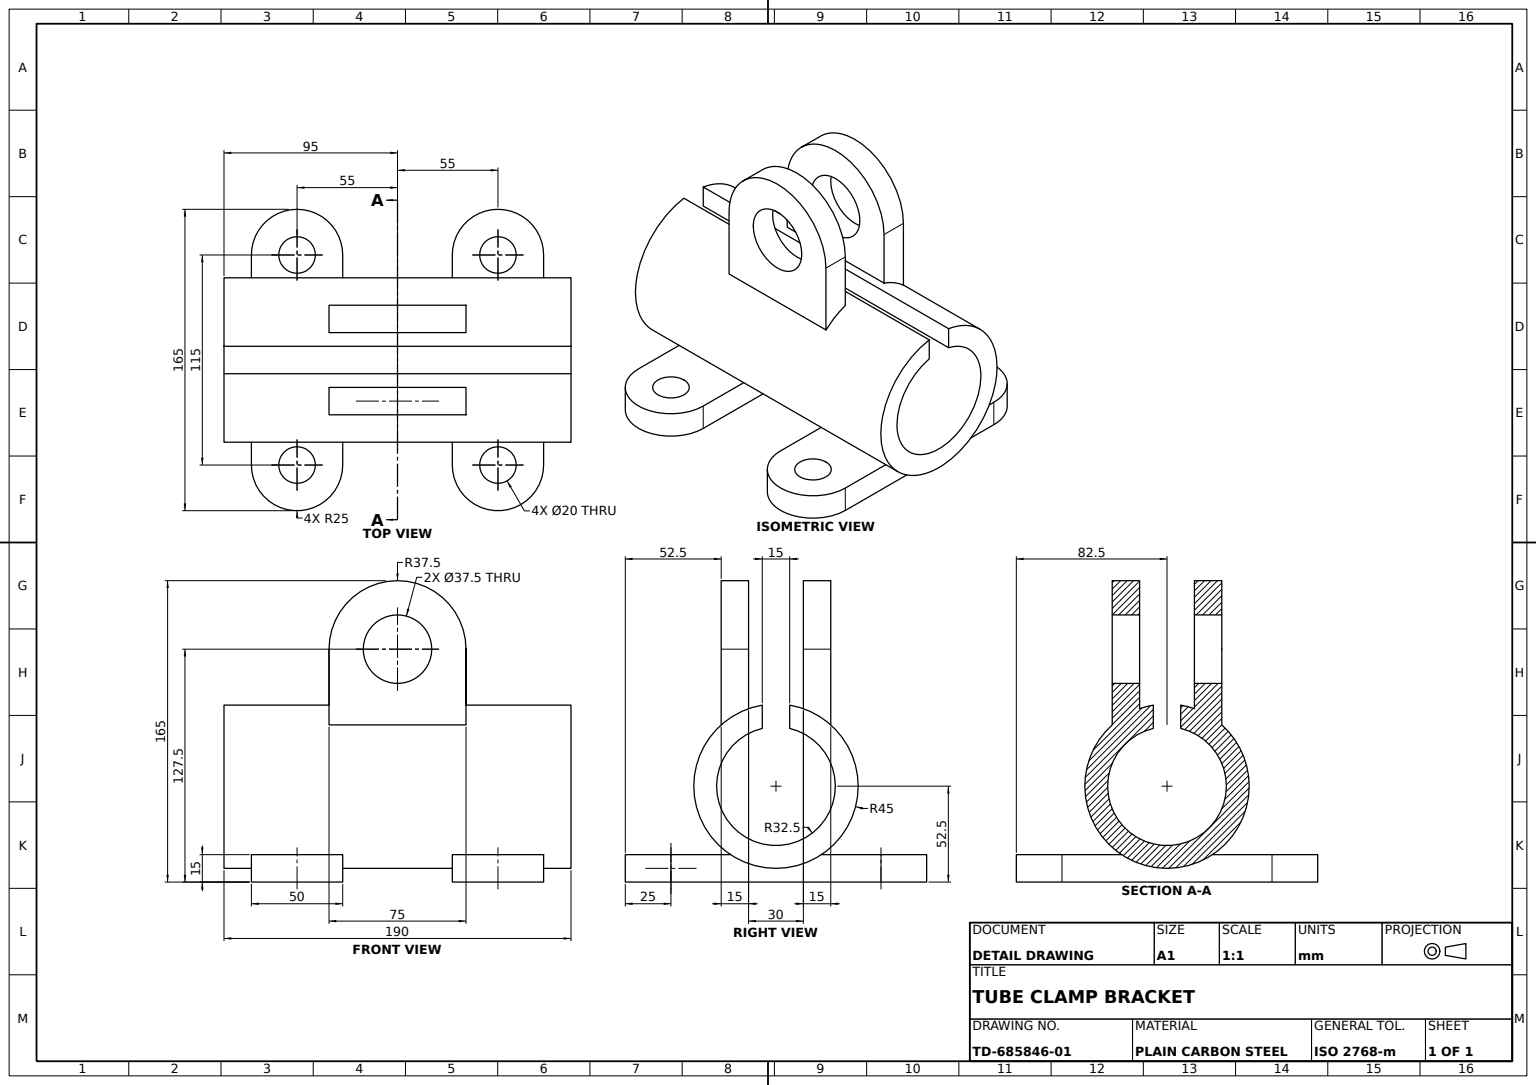
from build123d import *

# Parameters (mm, degrees)
SPLIT_SLEEVE_DEPTH                 = 95
SADDLE_BASE_PROFILE_W              = 50
SADDLE_BASE_PROFILE_H              = 15
SADDLE_BASE_DEPTH                  = 57.5
FOOT_TAB_DEPTH                     = 15
FOOT_TAB_MIRROR_RIGHT_COPY_1_DEPTH = 15
FOOT_MOUNTING_HOLES_4X_REACH       = 160.793
FOOT_HOLE_PROFILE_R                = 10
CLAMP_LUG_PROFILE_R                = 18.75
CLAMP_LUG_DEPTH                    = 15


with BuildPart() as part:
    # Split Sleeve Profile → Split Sleeve (new, symmetric)
    with BuildSketch(Plane(origin=(0, 0, 0), x_dir=(0, 0, -1), z_dir=(1, 0, 0))):
        with BuildLine():
            Line((-7.5, 44.370598373), (-7.5, 31.622776602))
            ThreePointArc((-7.5, 31.622776602), (0, -32.5), (7.5, 31.622776602))
            Line((7.5, 31.622776602), (7.5, 44.370598373))
            ThreePointArc((7.5, 44.370598373), (0, -45), (-7.5, 44.370598373))
        make_face()
    extrude(amount=SPLIT_SLEEVE_DEPTH, both=True)

    # Saddle Base Profile → Saddle Base (add, symmetric)
    with BuildSketch(Plane.XY):
        with Locations((-55, -45)):
            Rectangle(SADDLE_BASE_PROFILE_W, SADDLE_BASE_PROFILE_H)
        with Locations((55, -45)):
            Rectangle(SADDLE_BASE_PROFILE_W, SADDLE_BASE_PROFILE_H)
    extrude(amount=SADDLE_BASE_DEPTH, both=True)

    # Foot Tab Profile → Foot Tab (add)
    with BuildSketch(Plane.XZ.offset(52.5)):
        with BuildLine():
            Line((-80, 57.5), (-30, 57.5))
            ThreePointArc((-30, 57.5), (-55, 82.5), (-80, 57.5))
        make_face()
    foot_tab = extrude(amount=-FOOT_TAB_DEPTH)

    # Foot Tab Mirror Front: Foot Tab across plane
    add(foot_tab.mirror(Plane.XY))

    # Foot Tab Mirror Right: Foot Tab across plane
    add(foot_tab.mirror(Plane(origin=(0, 0, 0), x_dir=(0, 0, 1), z_dir=(1, 0, 0))))

    # Foot Tab Mirror Right copy 1 sketch → Foot Tab Mirror Right copy 1 (add)
    with BuildSketch(Plane(origin=(0, -52.5, 0), x_dir=(-1, 0, 0), z_dir=(0, -1, 0))):
        with BuildLine():
            Line((-80, 57.5), (-30, 57.5))
            ThreePointArc((-30, 57.5), (-55, 82.5), (-80, 57.5))
        make_face()
    extrude(amount=-FOOT_TAB_MIRROR_RIGHT_COPY_1_DEPTH)

    # Foot Hole Profile → Foot Mounting Holes 4x (cut, up to next)
    with BuildSketch(Plane.XZ.offset(52.5), mode=Mode.PRIVATE) as foot_mounting_holes_4x_sk1:
        with Locations(Location((-55, 57.5, 0), (0, 0, 270))):
            Circle(FOOT_HOLE_PROFILE_R)
    foot_mounting_holes_4x_tool1 = extrude(foot_mounting_holes_4x_sk1.sketch, amount=-FOOT_MOUNTING_HOLES_4X_REACH, mode=Mode.PRIVATE) & part.part
    # Foot Hole Profile → Foot Mounting Holes 4x (cut, up to next)
    with BuildSketch(Plane.XZ.offset(52.5), mode=Mode.PRIVATE) as foot_mounting_holes_4x_sk2:
        with Locations(Location((-55, -57.5, 0), (0, 0, 270))):
            Circle(FOOT_HOLE_PROFILE_R)
    foot_mounting_holes_4x_tool2 = extrude(foot_mounting_holes_4x_sk2.sketch, amount=-FOOT_MOUNTING_HOLES_4X_REACH, mode=Mode.PRIVATE) & part.part
    # Foot Hole Profile → Foot Mounting Holes 4x (cut, up to next)
    with BuildSketch(Plane.XZ.offset(52.5), mode=Mode.PRIVATE) as foot_mounting_holes_4x_sk3:
        with Locations(Location((55, -57.5, 0), (0, 0, 270))):
            Circle(FOOT_HOLE_PROFILE_R)
    foot_mounting_holes_4x_tool3 = extrude(foot_mounting_holes_4x_sk3.sketch, amount=-FOOT_MOUNTING_HOLES_4X_REACH, mode=Mode.PRIVATE) & part.part
    # Foot Hole Profile → Foot Mounting Holes 4x (cut, up to next)
    with BuildSketch(Plane.XZ.offset(52.5), mode=Mode.PRIVATE) as foot_mounting_holes_4x_sk4:
        with Locations(Location((55, 57.5, 0), (0, 0, 270))):
            Circle(FOOT_HOLE_PROFILE_R)
    foot_mounting_holes_4x_tool4 = extrude(foot_mounting_holes_4x_sk4.sketch, amount=-FOOT_MOUNTING_HOLES_4X_REACH, mode=Mode.PRIVATE) & part.part
    add(foot_mounting_holes_4x_tool1.solids().sort_by_distance((-55, -52.5, 57.5))[0], mode=Mode.SUBTRACT)
    add(foot_mounting_holes_4x_tool2.solids().sort_by_distance((-55, -52.5, -57.5))[0], mode=Mode.SUBTRACT)
    add(foot_mounting_holes_4x_tool3.solids().sort_by_distance((55, -52.5, -57.5))[0], mode=Mode.SUBTRACT)
    add(foot_mounting_holes_4x_tool4.solids().sort_by_distance((55, -52.5, 57.5))[0], mode=Mode.SUBTRACT)

    # Clamp Lug Profile → Clamp Lug (add)
    with BuildSketch(Plane.XY.offset(15)):
        with BuildLine():
            Line((-37.5, 75), (-37.5, 31.622776602))
            Line((-37.5, 31.622776602), (37.5, 31.622776602))
            Line((37.5, 31.622776602), (37.5, 75))
            ThreePointArc((37.5, 75), (0, 112.5), (-37.5, 75))
        make_face()
        with Locations((0, 75)):
            Circle(CLAMP_LUG_PROFILE_R, mode=Mode.SUBTRACT)
    clamp_lug = extrude(amount=CLAMP_LUG_DEPTH)

    # Clamp Lug Mirror: Clamp Lug across plane
    add(clamp_lug.mirror(Plane.XY))


solid = part.part
